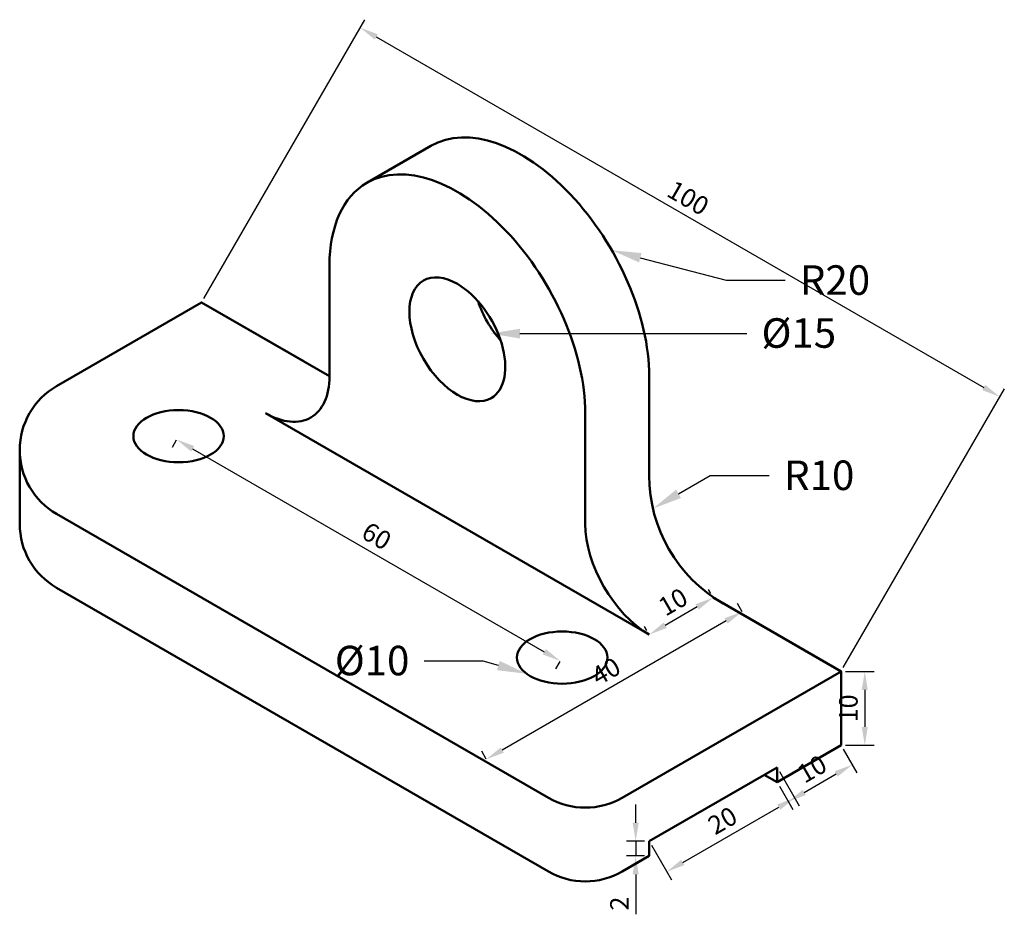
# Model space of a CAD drawing. Units: millimetres. Extents: x 2646 to 2779, y 1457 to 1579.
import ezdxf
from ezdxf import colors
from ezdxf.entities.mleader import LeaderData, LeaderLine
from ezdxf.math import Vec2, Vec3

# ---------------------------------------------------------------- set-up
doc = ezdxf.new("R2010")
doc.units = ezdxf.units.MM
for name, color, linetype, lineweight in [('M-DIMS', 2, 'Continuous', 25), ('M-OUTL', 7, 'Continuous', 50), ('M-TEXT', 3, 'Continuous', 25)]:
    doc.layers.add(name, color=color, linetype=linetype, lineweight=lineweight)
doc.styles.get("Standard").update_dxf_attribs({"font": 'arial.ttf'})
doc.dimstyles.new('ISO-25', dxfattribs={"dimtxt": 2.5, "dimasz": 2.5, "dimexe": 1.25, "dimexo": 0.625, "dimtad": 1, "dimtxsty": 'Standard', "dimcen": 2.5, "dimadec": 0, "dimazin": 0, "dimtfac": 1, "dimtmove": 0, "dimatfit": 3, "dimfxl": 1, "dimarcsym": 0})

# ---------------------------------------------------------------- blocks, each defined once
blk = doc.blocks.new('*D1')
at = {"layer": 'Defpoints', "color": 0, "transparency": 16777216}
for p in [(2739.92, 1500.34), (2731.26, 1495.34), (2731.26, 1495.34)]:
    blk.add_point(p, dxfattribs=at)
at = {"layer": 'M-DIMS', "color": 0, "lineweight": -2, "transparency": 16777216}
for p, q in [((2739.61, 1500.89), (2739.29, 1501.43)), ((2737.75, 1499.09), (2733.42, 1496.59)), ((2730.95, 1495.89), (2730.63, 1496.43))]:
    blk.add_line(p, q, dxfattribs=at)
at = {"layer": 'M-DIMS', "color": 0, "transparency": 16777216}
for points in [[(2737.55, 1499.46), (2737.96, 1498.73), (2739.92, 1500.34)], [(2733.21, 1496.96), (2733.63, 1496.23), (2731.26, 1495.34)]]:
    blk.add_solid(points, dxfattribs=at)
at = {"layer": 'M-DIMS', "color": 0, "transparency": 16777216, "insert": (2734.64, 1499.49), "char_height": 2.5, "attachment_point": 5, "rotation": 30}
blk.add_mtext('10', dxfattribs=at)
blk = doc.blocks.new('*D2')
at = {"layer": 'Defpoints', "color": 0, "transparency": 16777216}
for p in [(2667.52, 1522.22), (2719.21, 1491.77), (2719.48, 1492.22)]:
    blk.add_point(p, dxfattribs=at)
at = {"layer": 'M-DIMS', "color": 0, "lineweight": -2, "transparency": 16777216}
for p, q in [((2667.2, 1521.68), (2666.63, 1520.68)), ((2669.42, 1520.52), (2717.05, 1493.02)), ((2719.16, 1491.68), (2718.59, 1490.68))]:
    blk.add_line(p, q, dxfattribs=at)
at = {"layer": 'M-DIMS', "color": 0, "transparency": 16777216}
for points in [[(2669.63, 1520.88), (2669.21, 1520.15), (2667.25, 1521.77)], [(2717.26, 1493.38), (2716.84, 1492.65), (2719.21, 1491.77)]]:
    blk.add_solid(points, dxfattribs=at)
at = {"layer": 'M-DIMS', "color": 0, "transparency": 16777216, "insert": (2694.18, 1508.41), "char_height": 2.5, "attachment_point": 5, "rotation": 330}
blk.add_mtext('60', dxfattribs=at)
blk = doc.blocks.new('*D3')
at = {"layer": 'Defpoints', "color": 0, "transparency": 16777216}
for p in [(2757.24, 1480.34), (2758.76, 1477.71), (2748.58, 1475.34)]:
    blk.add_point(p, dxfattribs=at)
at = {"layer": 'M-DIMS', "color": 0, "lineweight": -2, "transparency": 16777216}
for p, q in [((2757.55, 1479.8), (2759.38, 1476.63)), ((2752.26, 1473.96), (2756.59, 1476.46)), ((2748.89, 1474.8), (2750.72, 1471.63))]:
    blk.add_line(p, q, dxfattribs=at)
at = {"layer": 'M-DIMS', "color": 0, "transparency": 16777216}
for points in [[(2756.38, 1476.82), (2756.8, 1476.1), (2758.76, 1477.71)], [(2752.05, 1474.32), (2752.47, 1473.6), (2750.1, 1472.71)]]:
    blk.add_solid(points, dxfattribs=at)
at = {"layer": 'M-DIMS', "color": 0, "transparency": 16777216, "insert": (2753.48, 1476.86), "char_height": 2.5, "attachment_point": 5, "rotation": 30}
blk.add_mtext('10', dxfattribs=at)
blk = doc.blocks.new('*D4')
at = {"layer": 'Defpoints', "color": 0, "transparency": 16777216}
for p in [(2748.58, 1477.34), (2750.96, 1473.21), (2731.26, 1467.34)]:
    blk.add_point(p, dxfattribs=at)
at = {"layer": 'M-DIMS', "color": 0, "lineweight": -2, "transparency": 16777216}
for p, q in [((2748.89, 1476.8), (2751.59, 1472.13)), ((2735.81, 1464.46), (2748.8, 1471.96)), ((2731.57, 1466.8), (2734.27, 1462.13))]:
    blk.add_line(p, q, dxfattribs=at)
at = {"layer": 'M-DIMS', "color": 0, "transparency": 16777216}
for points in [[(2748.59, 1472.32), (2749.01, 1471.6), (2750.96, 1473.21)], [(2735.6, 1464.82), (2736.02, 1464.1), (2733.64, 1463.21)]]:
    blk.add_solid(points, dxfattribs=at)
at = {"layer": 'M-DIMS', "color": 0, "transparency": 16777216, "insert": (2741.35, 1469.86), "char_height": 2.5, "attachment_point": 5, "rotation": 30}
blk.add_mtext('20', dxfattribs=at)
blk = doc.blocks.new('*D5')
at = {"layer": 'Defpoints', "color": 0, "transparency": 16777216}
for p in [(2757.24, 1490.34), (2757.24, 1480.34), (2760.46, 1480.34)]:
    blk.add_point(p, dxfattribs=at)
at = {"layer": 'M-DIMS', "color": 0, "lineweight": -2, "transparency": 16777216}
for p, q in [((2757.86, 1490.34), (2761.71, 1490.34)), ((2760.46, 1487.84), (2760.46, 1482.84)), ((2757.86, 1480.34), (2761.71, 1480.34))]:
    blk.add_line(p, q, dxfattribs=at)
at = {"layer": 'M-DIMS', "color": 0, "transparency": 16777216}
for points in [[(2760.04, 1487.84), (2760.87, 1487.84), (2760.46, 1490.34)], [(2760.04, 1482.84), (2760.87, 1482.84), (2760.46, 1480.34)]]:
    blk.add_solid(points, dxfattribs=at)
at = {"layer": 'M-DIMS', "color": 0, "transparency": 16777216, "insert": (2758.56, 1485.34), "char_height": 2.5, "attachment_point": 5, "rotation": 90}
blk.add_mtext('10', dxfattribs=at)
blk = doc.blocks.new('*D6')
at = {"layer": 'Defpoints', "color": 0, "transparency": 16777216}
for p in [(2670.64, 1540.34), (2778.73, 1527.57), (2757.24, 1490.34)]:
    blk.add_point(p, dxfattribs=at)
at = {"layer": 'M-DIMS', "color": 0, "lineweight": -2, "transparency": 16777216}
for p, q in [((2670.95, 1540.89), (2692.75, 1578.65)), ((2694.29, 1576.32), (2776.57, 1528.82)), ((2757.55, 1490.89), (2779.36, 1528.65))]:
    blk.add_line(p, q, dxfattribs=at)
at = {"layer": 'M-DIMS', "color": 0, "transparency": 16777216}
for points in [[(2694.5, 1576.68), (2694.09, 1575.96), (2692.13, 1577.57)], [(2776.77, 1529.18), (2776.36, 1528.46), (2778.73, 1527.57)]]:
    blk.add_solid(points, dxfattribs=at)
at = {"layer": 'M-DIMS', "color": 0, "transparency": 16777216, "insert": (2736.38, 1554.22), "char_height": 2.5, "attachment_point": 5, "rotation": 330}
blk.add_mtext('100', dxfattribs=at)
blk = doc.blocks.new('*D7')
at = {"layer": 'Defpoints', "color": 0, "transparency": 16777216}
for p in [(2744.15, 1497.9), (2709.19, 1478.44), (2709.51, 1477.9)]:
    blk.add_point(p, dxfattribs=at)
at = {"layer": 'M-DIMS', "color": 0, "lineweight": -2, "transparency": 16777216}
for p, q in [((2743.83, 1498.44), (2743.21, 1499.53)), ((2741.67, 1497.19), (2711.36, 1479.69)), ((2709.19, 1478.44), (2708.57, 1479.53))]:
    blk.add_line(p, q, dxfattribs=at)
at = {"layer": 'M-DIMS', "color": 0, "transparency": 16777216}
for points in [[(2741.46, 1497.55), (2741.88, 1496.83), (2743.84, 1498.44)], [(2711.15, 1480.05), (2711.57, 1479.33), (2709.19, 1478.44)]]:
    blk.add_solid(points, dxfattribs=at)
at = {"layer": 'M-DIMS', "color": 0, "transparency": 16777216, "insert": (2725.56, 1490.09), "char_height": 2.5, "attachment_point": 5, "rotation": 30}
blk.add_mtext('40', dxfattribs=at)
blk = doc.blocks.new('*D8')
at = {"layer": 'Defpoints', "color": 0, "transparency": 16777216}
for p in [(2731.26, 1467.34), (2729.43, 1465.34), (2731.26, 1465.34)]:
    blk.add_point(p, dxfattribs=at)
at = {"layer": 'M-DIMS', "color": 0, "lineweight": -2, "transparency": 16777216}
for p, q in [((2729.43, 1469.84), (2729.43, 1472.34)), ((2730.63, 1467.34), (2728.18, 1467.34)), ((2729.43, 1467.34), (2729.43, 1465.34)), ((2730.63, 1465.34), (2728.18, 1465.34)), ((2729.43, 1462.84), (2729.43, 1457.44))]:
    blk.add_line(p, q, dxfattribs=at)
at = {"layer": 'M-DIMS', "color": 0, "transparency": 16777216}
for points in [[(2729.01, 1469.84), (2729.84, 1469.84), (2729.43, 1467.34)], [(2729.01, 1462.84), (2729.84, 1462.84), (2729.43, 1465.34)]]:
    blk.add_solid(points, dxfattribs=at)
at = {"layer": 'M-DIMS', "color": 0, "transparency": 16777216, "insert": (2727.55, 1458.89), "char_height": 2.5, "attachment_point": 5, "rotation": 90}
blk.add_mtext('2', dxfattribs=at)

msp = doc.modelspace()

# ---------------------------------------------------------------- linework, layer by layer
at = {"layer": 'M-OUTL'}
for p, q in [((2701.69, 1561.557), (2693.03, 1556.557)), ((2687.957, 1545.343), (2687.957, 1530.343)), ((2687.957, 1530.343), (2670.636, 1540.343)), ((2731.258, 1530.344), (2731.258, 1516.891)), ((2679.296, 1525.343), (2731.258, 1495.343)), ((2722.598, 1510.343), (2722.598, 1525.343)), ((2645.995, 1510.344), (2645.995, 1520.344)), ((2757.239, 1480.344), (2757.239, 1490.344)), ((2757.239, 1480.344), (2748.579, 1475.344)), ((2748.579, 1477.344), (2731.258, 1467.344)), ((2748.578, 1475.343), (2746.846, 1476.343)), ((2748.579, 1475.344), (2748.579, 1477.344)), ((2731.258, 1467.344), (2731.258, 1465.344))]:
    msp.add_line(p, q, dxfattribs=at)
for points in [[(2684.53, 1532.323), (2670.636, 1540.344), (2650.995, 1529.005, 0.5773503), (2650.995, 1511.684), (2717.598, 1473.231, 0.2679492), (2727.598, 1473.231), (2757.239, 1490.344), (2739.918, 1500.344)], [(2645.995, 1510.344, 0.2679492), (2650.995, 1501.684), (2717.598, 1463.231, 0.2679492), (2727.598, 1463.231), (2731.258, 1465.344)]]:
    msp.add_lwpolyline(points, format="xyb", dxfattribs=at)
msp.add_lwpolyline([(2748.579, 1475.344), (2757.239, 1480.344)], dxfattribs=at)
msp.add_arc((2751.258, 1516.891), 20, 180, 240, dxfattribs=at)
for centre, major_axis, start_param, end_param in [((2713.938, 1540.344), (12.247, -21.213), 0.7853982, 3.1415927), ((2705.277, 1535.343), (-12.247, 21.213), 3.9269908, 6.2831853), ((2705.277, 1535.343), (-12.247, 21.213), 0, 0.7853982), ((2705.277, 1535.343), (4.593, -7.955), 3.1415927, 6.2831853), ((2705.277, 1535.343), (4.593, -7.955), 2.3561945, 3.1415927), ((2705.277, 1535.343), (4.593, -7.955), 0, 2.3561945), ((2713.937, 1540.343), (4.593, -7.955), 4.3725521, 5.0522259), ((2679.296, 1535.344), (6.124, -10.607), 0, 0.785375), ((2679.296, 1535.344), (6.124, -10.607), 5.4978103, 6.2831853), ((2731.258, 1505.344), (6.124, -10.607), 3.927014, 5.497764)]:
    msp.add_ellipse(centre, major_axis=major_axis, ratio=0.5773503, start_param=start_param, end_param=end_param, dxfattribs=at)
for centre in [(2667.516, 1522.223), (2719.477, 1492.223)]:
    msp.add_ellipse(centre, major_axis=(-6.124, 0), ratio=0.5773503, dxfattribs=at)

# ---------------------------------------------------------------- dimensions: what is measured, and where the dimension line sits
at = {"layer": 'M-DIMS'}
for p1, p2, distance, picture, middle in [((2670.636, 1540.344), (2757.239, 1490.344), 42.985, '*D6', (2736.381, 1554.217)), ((2667.516, 1522.223), (2719.477, 1492.223), -0.528, '*D2', (2694.183, 1508.412)), ((2739.918, 1500.344), (2731.258, 1495.344), 0, '*D1', (2734.638, 1499.491)), ((2744.147, 1497.903), (2709.506, 1477.903), -0.623, '*D7', (2725.564, 1490.089)), ((2757.239, 1490.344), (2757.239, 1480.344), 3.219, '*D5', (2758.556, 1485.344)), ((2748.579, 1475.344), (2757.239, 1480.344), -3.037, '*D3', (2753.477, 1476.861)), ((2731.258, 1467.344), (2748.579, 1477.344), -4.769, '*D4', (2741.352, 1469.861)), ((2731.258, 1467.344), (2731.258, 1465.344), -1.83, '*D8', (2727.548, 1458.892))]:
    dim = msp.add_aligned_dim(p1=p1, p2=p2, distance=distance, dimstyle='ISO-25', override={"dimclrd": 0, "dimclre": 0, "dimclrt": 0}, dxfattribs=at)
    dim.commit()
    dim.dimension.update_dxf_attribs({"geometry": picture, "text_midpoint": middle})

# ---------------------------------------------------------------- leaders
at = {"layer": 'M-TEXT'}
ml = msp.add_multileader_mtext('Standard', dxfattribs=at)
ml.set_content('R20', color=256)
ml.set_leader_properties()
ml.build(insert=Vec2(0, 0))
ctx = ml.context
ctx.base_point, ctx.plane_origin = Vec3(2749.662, 1543.34), Vec3(2726.185, 1547.416)
notes = []
notes.append((ctx, [(0, (1, 1, 0), (2741.662, 1543.34), (1, 0), 8, [(0, [(2726.185, 1547.416)], 0, [])])]))
ctx.mtext.insert, ctx.mtext.flow_direction = Vec3(2751.662, 1545.374), 5
ml = msp.add_multileader_mtext('Standard', dxfattribs=at)
ml.set_content('%%C15', color=256)
ml.set_leader_properties()
ml.build(insert=Vec2(0, 0))
ctx = ml.context
ctx.base_point, ctx.plane_origin = Vec3(2744.472, 1536.118), Vec3(2709.747, 1536.118)
notes.append((ctx, [(0, (1, 1, 0), (2736.472, 1536.118), (1, 0), 8, [(0, [(2709.747, 1536.118)], 0, [])])]))
ctx.mtext.insert, ctx.mtext.flow_direction = Vec3(2746.472, 1538.198), 5
ml = msp.add_multileader_mtext('Standard', dxfattribs=at)
ml.set_content('R10', color=256)
ml.set_leader_properties()
ml.build(insert=Vec2(0, 0))
ctx = ml.context
ctx.base_point, ctx.plane_origin = Vec3(2747.524, 1516.891), Vec3(2731.766, 1512.412)
notes.append((ctx, [(0, (1, 1, 0), (2739.524, 1516.891), (1, 0), 8, [(0, [(2731.766, 1512.412)], 0, [])])]))
ctx.mtext.insert, ctx.mtext.flow_direction = Vec3(2749.524, 1518.926), 5
ml = msp.add_multileader_mtext('Standard', dxfattribs=at)
ml.set_content('%%C10', color=256)
ml.set_leader_properties()
ml.build(insert=Vec2(0, 0))
ctx = ml.context
ctx.base_point, ctx.plane_origin = Vec3(2686.71, 1491.739), Vec3(2714.679, 1490.026)
ctx.text_align_type = 2
notes.append((ctx, [(0, (1, 1, 0), (2708.778, 1491.739), (-1, 0), 8, [(0, [(2714.679, 1490.026)], 0, [])])]))
ctx.mtext.insert, ctx.mtext.alignment, ctx.mtext.flow_direction = Vec3(2698.778, 1493.819), 3, 5
for ctx, leaders in notes:
    for number, flags, end, landing, length, lines in leaders:
        leader = LeaderData()
        leader.index, (leader.has_last_leader_line, leader.has_dogleg_vector, leader.attachment_direction) = number, flags
        leader.last_leader_point, leader.dogleg_vector, leader.dogleg_length = Vec3(end), Vec3(landing), length
        for number, points, colour, breaks in lines:
            line = LeaderLine()
            line.index, line.vertices, line.color, line.breaks = number, Vec3.list(points), colors.encode_raw_color(colour), breaks
            leader.lines.append(line)
        ctx.leaders.append(leader)

doc.saveas('drawing.dxf')
